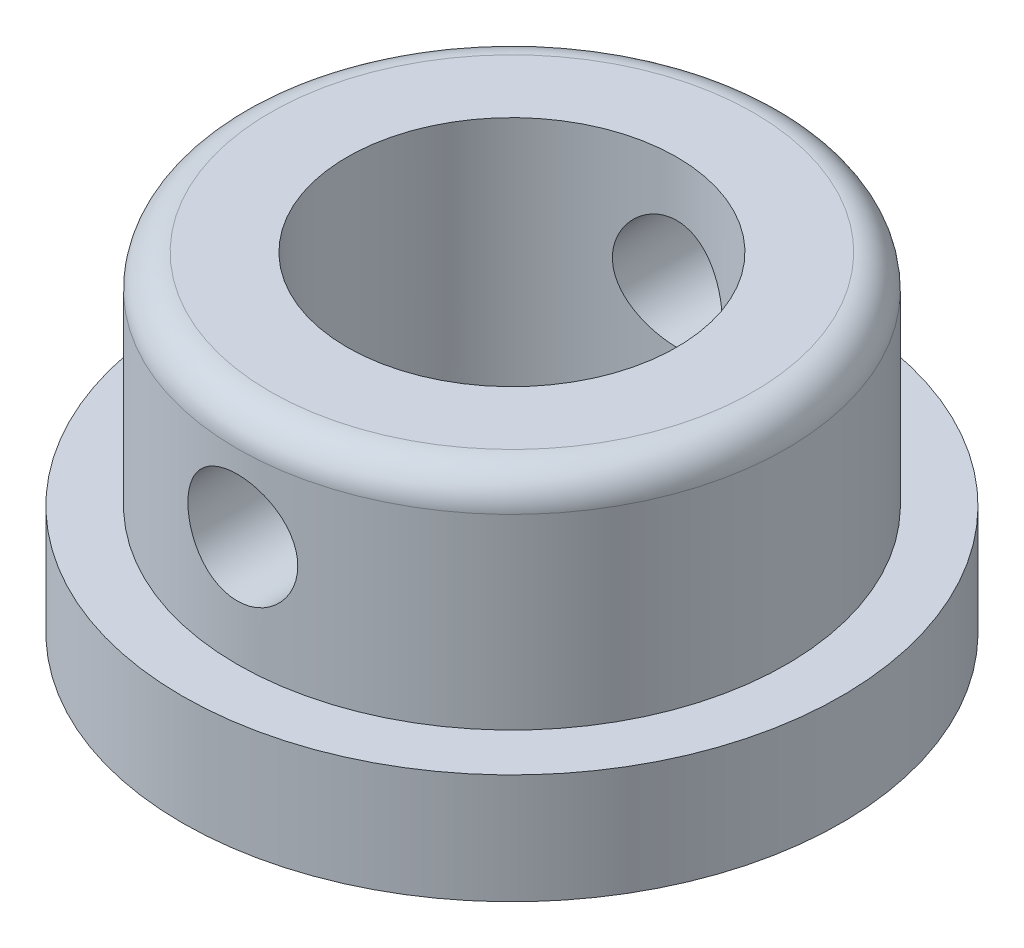
ISO-10303-21;
HEADER;
FILE_DESCRIPTION(('STEP AP214'),'2;1');
FILE_NAME('part.step','',(''),(''),'','','');
FILE_SCHEMA(('AUTOMOTIVE_DESIGN { 1 0 10303 214 1 1 1 1 }'));
ENDSEC;
DATA;
#1=APPLICATION_CONTEXT('core data for automotive mechanical design processes');
#2=APPLICATION_PROTOCOL_DEFINITION('international standard','automotive_design',2000,#1);
#3=PRODUCT_CONTEXT('',#1,'mechanical');
#4=PRODUCT('Part','Part','',(#3));
#5=PRODUCT_RELATED_PRODUCT_CATEGORY('part','',(#4));
#6=PRODUCT_DEFINITION_FORMATION('','',#4);
#7=PRODUCT_DEFINITION_CONTEXT('part definition',#1,'design');
#8=PRODUCT_DEFINITION('design','',#6,#7);
#9=PRODUCT_DEFINITION_SHAPE('','',#8);
#10=(LENGTH_UNIT() NAMED_UNIT(*) SI_UNIT(.MILLI.,.METRE.));
#11=(NAMED_UNIT(*) PLANE_ANGLE_UNIT() SI_UNIT($,.RADIAN.));
#12=(NAMED_UNIT(*) SI_UNIT($,.STERADIAN.) SOLID_ANGLE_UNIT());
#13=UNCERTAINTY_MEASURE_WITH_UNIT(LENGTH_MEASURE(1.E-05),#10,'distance_accuracy_value','');
#14=(GEOMETRIC_REPRESENTATION_CONTEXT(3) GLOBAL_UNCERTAINTY_ASSIGNED_CONTEXT((#13)) GLOBAL_UNIT_ASSIGNED_CONTEXT((#10,
#11,#12)) REPRESENTATION_CONTEXT('',''));
#15=CARTESIAN_POINT('',(0.,0.,0.));
#16=DIRECTION('',(0.,0.,1.));
#17=DIRECTION('',(1.,0.,0.));
#18=AXIS2_PLACEMENT_3D('',#15,#16,#17);
#19=CARTESIAN_POINT('',(0.,20.,-35.));
#20=DIRECTION('',(0.,0.,1.));
#21=DIRECTION('',(1.,0.,0.));
#22=AXIS2_PLACEMENT_3D('',#19,#20,#21);
#23=CYLINDRICAL_SURFACE('',#22,5.);
#24=CARTESIAN_POINT('',(5.,20.,-14.142135623731));
#25=CARTESIAN_POINT('',(5.00000128973857,20.2723408741804,-14.1421347265217));
#26=CARTESIAN_POINT('',(4.97767391842761,20.544673999118,-14.1500884645429));
#27=CARTESIAN_POINT('',(4.88925565844404,21.0812721049712,-14.1808787040627));
#28=CARTESIAN_POINT('',(4.82315756084199,21.3455357493623,-14.2037176571094));
#29=CARTESIAN_POINT('',(4.64977742842453,21.8581344649864,-14.2614101844396));
#30=CARTESIAN_POINT('',(4.54257610701623,22.1064996472136,-14.2962401985661));
#31=CARTESIAN_POINT('',(4.29030814220691,22.5818002427398,-14.3739561005162));
#32=CARTESIAN_POINT('',(4.14523314430092,22.8087309127682,-14.4168437651806));
#33=CARTESIAN_POINT('',(3.81525573221439,23.2435998116916,-14.5077244703737));
#34=CARTESIAN_POINT('',(3.6291217068896,23.4505771433586,-14.5558447422322));
#35=CARTESIAN_POINT('',(3.22493833607198,23.8310340061232,-14.6506932400501));
#36=CARTESIAN_POINT('',(3.00688387526188,24.0045081579118,-14.6974212414481));
#37=CARTESIAN_POINT('',(2.53802253982505,24.317394486648,-14.7856933460899));
#38=CARTESIAN_POINT('',(2.28650955612262,24.4557998530898,-14.8270703850803));
#39=CARTESIAN_POINT('',(1.76215611493737,24.6879579256375,-14.8984793385491));
#40=CARTESIAN_POINT('',(1.48932142843606,24.7817226658845,-14.9285143101501));
#41=CARTESIAN_POINT('',(0.940144087167472,24.918679273162,-14.9729537715953));
#42=CARTESIAN_POINT('',(0.664253774264842,24.963517231285,-14.987865738878));
#43=CARTESIAN_POINT('',(0.108489374120447,25.0065814668033,-15.0021804109124));
#44=CARTESIAN_POINT('',(-0.171383667719483,25.0048197582621,-15.0015871131448));
#45=CARTESIAN_POINT('',(-0.715517575969074,24.9557787271699,-14.9853019809366));
#46=CARTESIAN_POINT('',(-0.979960242958283,24.9102873576276,-14.9702032377559));
#47=CARTESIAN_POINT('',(-1.49721719411086,24.7780350950976,-14.9273483669866));
#48=CARTESIAN_POINT('',(-1.75003068889608,24.6912714051009,-14.8995913815591));
#49=CARTESIAN_POINT('',(-2.24076237420987,24.4778934134697,-14.8337835146612));
#50=CARTESIAN_POINT('',(-2.47844110484423,24.3507703072674,-14.7956021262008));
#51=CARTESIAN_POINT('',(-2.92962162763661,24.0607014727567,-14.712919651946));
#52=CARTESIAN_POINT('',(-3.14311667192671,23.8977457833618,-14.6684168100733));
#53=CARTESIAN_POINT('',(-3.55050433275654,23.5316280327015,-14.5753095924948));
#54=CARTESIAN_POINT('',(-3.74300078532636,23.3269342107926,-14.5266107584439));
#55=CARTESIAN_POINT('',(-4.09138629799087,22.8877563713669,-14.432366762445));
#56=CARTESIAN_POINT('',(-4.24726971640772,22.6532677713598,-14.3868220872808));
#57=CARTESIAN_POINT('',(-4.51993727517872,22.1567318719828,-14.3035262560556));
#58=CARTESIAN_POINT('',(-4.6361323181067,21.8943393434111,-14.2658954642374));
#59=CARTESIAN_POINT('',(-4.82221596634668,21.3521430289279,-14.2040825412192));
#60=CARTESIAN_POINT('',(-4.89212397873747,21.0723465939688,-14.1798947743546));
#61=CARTESIAN_POINT('',(-4.98080641048761,20.5168082229421,-14.1489818157793));
#62=CARTESIAN_POINT('',(-5.00174547753816,20.2414528762567,-14.1415180159378));
#63=CARTESIAN_POINT('',(-4.9980271945486,19.6911192544295,-14.1428336029592));
#64=CARTESIAN_POINT('',(-4.97337812613382,19.4161409198801,-14.1516100395907));
#65=CARTESIAN_POINT('',(-4.88112825776155,18.8842151714404,-14.183680904515));
#66=CARTESIAN_POINT('',(-4.81503196990342,18.6269728492458,-14.206466272042));
#67=CARTESIAN_POINT('',(-4.64356931280233,18.1272819688041,-14.2634276835511));
#68=CARTESIAN_POINT('',(-4.53819598181711,17.8848360420461,-14.297605746742));
#69=CARTESIAN_POINT('',(-4.28737170369468,17.413097895765,-14.3748438797893));
#70=CARTESIAN_POINT('',(-4.14075559179248,17.184466786791,-14.4181512832814));
#71=CARTESIAN_POINT('',(-3.81292815278779,16.7542697380814,-14.5082884365483));
#72=CARTESIAN_POINT('',(-3.63170662749391,16.5527118066939,-14.5551192221897));
#73=CARTESIAN_POINT('',(-3.22945852950163,16.1723600795468,-14.6497519318925));
#74=CARTESIAN_POINT('',(-3.00693635273326,15.9951280499057,-14.6974921788948));
#75=CARTESIAN_POINT('',(-2.53413645700128,15.6804192882598,-14.7863425806554));
#76=CARTESIAN_POINT('',(-2.28385972432276,15.5429411441879,-14.8274529708847));
#77=CARTESIAN_POINT('',(-1.76389931216148,15.3128994756914,-14.8982202905301));
#78=CARTESIAN_POINT('',(-1.49435561660598,15.2200436142597,-14.9279515002266));
#79=CARTESIAN_POINT('',(-0.942292329230079,15.0813612896995,-14.9729305418887));
#80=CARTESIAN_POINT('',(-0.659777459769445,15.0355178505975,-14.9881836017009));
#81=CARTESIAN_POINT('',(-0.104076679300203,14.9936896119718,-15.0020931618128));
#82=CARTESIAN_POINT('',(0.168923619600093,14.9954627303381,-15.001496004472));
#83=CARTESIAN_POINT('',(0.71055572500087,15.043286540732,-14.9856098259699));
#84=CARTESIAN_POINT('',(0.979187884095285,15.0893336407638,-14.9703219966788));
#85=CARTESIAN_POINT('',(1.5002105971603,15.2229111728798,-14.9270457477206));
#86=CARTESIAN_POINT('',(1.75279135456395,15.3097710767647,-14.8992629180574));
#87=CARTESIAN_POINT('',(2.23989175469898,15.5218876554858,-14.8338580352247));
#88=CARTESIAN_POINT('',(2.47440812071216,15.6471512759851,-14.7962342024008));
#89=CARTESIAN_POINT('',(2.92817008154393,15.93784756051,-14.713293441394));
#90=CARTESIAN_POINT('',(3.14653125778804,16.1045934269082,-14.6677436245963));
#91=CARTESIAN_POINT('',(3.55290513136214,16.471286955781,-14.574649439594));
#92=CARTESIAN_POINT('',(3.74090810812296,16.6712452113136,-14.5271044386549));
#93=CARTESIAN_POINT('',(4.08870904416559,17.1080467779347,-14.4331639912799));
#94=CARTESIAN_POINT('',(4.2471148299895,17.3460275548832,-14.3868863994315));
#95=CARTESIAN_POINT('',(4.52157171650558,17.8466721345139,-14.3030096661508));
#96=CARTESIAN_POINT('',(4.63763388409737,18.1093294651483,-14.2654082580625));
#97=CARTESIAN_POINT('',(4.81921914102083,18.6398091200782,-14.2050667103257));
#98=CARTESIAN_POINT('',(4.8867895457476,18.9068613176268,-14.1817316428591));
#99=CARTESIAN_POINT('',(4.97717160074634,19.4492802523335,-14.1502691769759));
#100=CARTESIAN_POINT('',(4.99999869598296,19.7246440870535,-14.1421365308731));
#101=CARTESIAN_POINT('',(5.,20.,-14.142135623731));
#102=B_SPLINE_CURVE_WITH_KNOTS('',3,(#24,#25,#26,#27,#28,#29,#30,#31,#32,#33,#34,#35,#36,#37,
#38,#39,#40,#41,#42,#43,#44,#45,#46,#47,#48,#49,#50,#51,#52,#53,#54,#55,#56,#57,#58,#59,#60,#61,
#62,#63,#64,#65,#66,#67,#68,#69,#70,#71,#72,#73,#74,#75,#76,#77,#78,#79,#80,#81,#82,#83,#84,#85,
#86,#87,#88,#89,#90,#91,#92,#93,#94,#95,#96,#97,#98,#99,#100,#101),.UNSPECIFIED.,.T.,.F.,(4,2,2,
2,2,2,2,2,2,2,2,2,2,2,2,2,2,2,2,2,2,2,2,2,2,2,2,2,2,2,2,2,2,2,2,2,2,2,4),(0.,0.816002923996784,
1.63214027507582,2.44668313750414,3.26140583092721,4.1050668713784,4.9488632585994,
5.81467530718286,6.68025381933945,7.51571593824671,8.35096266511636,9.15345024127845,
9.95599220946183,10.7690827430168,11.5823995937011,12.4340087181959,13.2857489806053,
14.1496319921528,15.0131525678308,15.837714568222,16.6621267918617,17.4582197884388,
18.2544539573473,19.0759428867857,19.8976742831064,20.7589404085546,21.6201759378766,
22.4756895595426,23.3308941502078,24.1459042338818,24.9608482004891,25.7628478020215,
26.5649925381621,27.3967759760317,28.2288252216316,29.0934451368072,29.9578389133433,
30.7831606081345,31.6081973595232),.UNSPECIFIED.);
#103=CARTESIAN_POINT('',(5.,20.,-14.142135623731));
#104=VERTEX_POINT('',#103);
#105=EDGE_CURVE('E50',#104,#104,#102,.T.);
#106=ORIENTED_EDGE('',*,*,#105,.T.);
#107=EDGE_LOOP('',(#106));
#108=FACE_BOUND('',#107,.T.);
#109=CARTESIAN_POINT('',(0.,25.,-25.));
#110=CARTESIAN_POINT('',(-0.138987493787324,25.0000027694463,-25.0000014065203));
#111=CARTESIAN_POINT('',(-0.277940302046088,24.9942032492811,-24.9988389427216));
#112=CARTESIAN_POINT('',(-0.554886864496204,24.9710563512974,-24.994224565157));
#113=CARTESIAN_POINT('',(-0.692880432791919,24.9537067948975,-24.9907722194715));
#114=CARTESIAN_POINT('',(-0.966937148503881,24.9075814377122,-24.981670242636));
#115=CARTESIAN_POINT('',(-1.10299928122357,24.8787998455141,-24.9760194978176));
#116=CARTESIAN_POINT('',(-1.37221108352448,24.810025349109,-24.9626762565998));
#117=CARTESIAN_POINT('',(-1.50535966309261,24.7700283237777,-24.9549830097359));
#118=CARTESIAN_POINT('',(-1.76758319373794,24.6791962522582,-24.9377804442932));
#119=CARTESIAN_POINT('',(-1.896663374225,24.6283758297848,-24.9282735779222));
#120=CARTESIAN_POINT('',(-2.15009997814349,24.5162240178123,-24.9076944208426));
#121=CARTESIAN_POINT('',(-2.2744546389337,24.4548887523412,-24.8966215531404));
#122=CARTESIAN_POINT('',(-2.51749782000809,24.3221945692906,-24.8732206370355));
#123=CARTESIAN_POINT('',(-2.63618884664852,24.2508401417061,-24.8608931515555));
#124=CARTESIAN_POINT('',(-2.86722020463686,24.0985603647523,-24.8353088041128));
#125=CARTESIAN_POINT('',(-2.97955814193969,24.0176314424647,-24.8220515959613));
#126=CARTESIAN_POINT('',(-3.1983785388143,23.8457711931702,-24.7948114657324));
#127=CARTESIAN_POINT('',(-3.30477652475173,23.7547333566458,-24.780821838943));
#128=CARTESIAN_POINT('',(-3.50958996762926,23.5640376679645,-24.7526457290753));
#129=CARTESIAN_POINT('',(-3.60800245195942,23.4643766340819,-24.738459174971));
#130=CARTESIAN_POINT('',(-3.79610927604841,23.2571655640739,-24.7102933832022));
#131=CARTESIAN_POINT('',(-3.8858061217282,23.1496178112366,-24.6963140869323));
#132=CARTESIAN_POINT('',(-4.05592901668139,22.9272928345424,-24.6689453876667));
#133=CARTESIAN_POINT('',(-4.13635163435981,22.8125129588355,-24.6555562041458));
#134=CARTESIAN_POINT('',(-4.28798741229219,22.5754841568505,-24.6296394657581));
#135=CARTESIAN_POINT('',(-4.35911381454495,22.4531786550123,-24.6171204770982));
#136=CARTESIAN_POINT('',(-4.49081269831453,22.2028712528765,-24.5934353082732));
#137=CARTESIAN_POINT('',(-4.55138122040544,22.0748672380124,-24.5822696361062));
#138=CARTESIAN_POINT('',(-4.71644727257975,21.6837416438572,-24.5513304070068));
#139=CARTESIAN_POINT('',(-4.8044888260482,21.4132193246056,-24.5340820165952));
#140=CARTESIAN_POINT('',(-4.93264780265691,20.8645385652061,-24.508635793463));
#141=CARTESIAN_POINT('',(-4.97337819482264,20.5865266702931,-24.5003223072134));
#142=CARTESIAN_POINT('',(-5.00775493418216,20.027461501124,-24.4933199482487));
#143=CARTESIAN_POINT('',(-5.00140609582258,19.7464085407904,-24.4946300913956));
#144=CARTESIAN_POINT('',(-4.94227436036826,19.1937632800715,-24.5066272442008));
#145=CARTESIAN_POINT('',(-4.89019310186595,18.9220922268258,-24.5171725589932));
#146=CARTESIAN_POINT('',(-4.7421890224497,18.3914203617583,-24.546227391949));
#147=CARTESIAN_POINT('',(-4.64626410780486,18.1324201556801,-24.5647372904543));
#148=CARTESIAN_POINT('',(-4.41262402680007,17.6324234898532,-24.6077809023025));
#149=CARTESIAN_POINT('',(-4.27463078523214,17.3915605480925,-24.632354484594));
#150=CARTESIAN_POINT('',(-3.96096784378848,16.9361458042038,-24.684730944745));
#151=CARTESIAN_POINT('',(-3.78529381392921,16.721597030353,-24.7125341935642));
#152=CARTESIAN_POINT('',(-3.39749968079915,16.3208529728437,-24.7688510603976));
#153=CARTESIAN_POINT('',(-3.18478080820446,16.1352371567135,-24.797368460096));
#154=CARTESIAN_POINT('',(-2.73092511816778,15.8022307724848,-24.8514424361697));
#155=CARTESIAN_POINT('',(-2.48978793632426,15.654840694624,-24.8769989745701));
#156=CARTESIAN_POINT('',(-1.98529693496818,15.4023624527765,-24.9223345079227));
#157=CARTESIAN_POINT('',(-1.72190909807365,15.2973405314029,-24.9421044423773));
#158=CARTESIAN_POINT('',(-1.18074488209619,15.1331976301815,-24.9735704494292));
#159=CARTESIAN_POINT('',(-0.9029702503472,15.0740710900358,-24.98526750005));
#160=CARTESIAN_POINT('',(-0.34589702815055,15.0042177306314,-24.9991335933204));
#161=CARTESIAN_POINT('',(-0.0667016415443239,14.9926979010851,-25.0014587325673));
#162=CARTESIAN_POINT('',(0.489624670880016,15.0162492959244,-24.9967525965614));
#163=CARTESIAN_POINT('',(0.766755711869967,15.0513179012196,-24.9897218472742));
#164=CARTESIAN_POINT('',(1.30852830007857,15.1663918633032,-24.9671916002008));
#165=CARTESIAN_POINT('',(1.57325974299468,15.2459903260944,-24.9517688194687));
#166=CARTESIAN_POINT('',(2.08561813620307,15.4474199296754,-24.9141776037933));
#167=CARTESIAN_POINT('',(2.33324380335236,15.5692542345549,-24.892008663478));
#168=CARTESIAN_POINT('',(2.80770587332562,15.853412391337,-24.8429955738642));
#169=CARTESIAN_POINT('',(3.03425065213174,16.0162136728006,-24.8160975113418));
#170=CARTESIAN_POINT('',(3.45709007722326,16.3770461884555,-24.760736752006));
#171=CARTESIAN_POINT('',(3.65338147605435,16.5750811997927,-24.7322738876682));
#172=CARTESIAN_POINT('',(4.01320302351496,17.0043658784477,-24.6764651380018));
#173=CARTESIAN_POINT('',(4.17618877400404,17.2360754097949,-24.6491428619003));
#174=CARTESIAN_POINT('',(4.46092683850573,17.7240601179627,-24.5992097395686));
#175=CARTESIAN_POINT('',(4.58268080227279,17.9803343113826,-24.5765987048474));
#176=CARTESIAN_POINT('',(4.78076018011429,18.5088289322538,-24.5388364729789));
#177=CARTESIAN_POINT('',(4.85732111853824,18.7809584178571,-24.5236466726876));
#178=CARTESIAN_POINT('',(4.96353963899985,19.3347130495845,-24.5023739077135));
#179=CARTESIAN_POINT('',(4.9932033375265,19.6163369525221,-24.4962897554484));
#180=CARTESIAN_POINT('',(5.00179339144585,20.0366703889551,-24.4945288792509));
#181=CARTESIAN_POINT('',(4.99885021968412,20.1752265681492,-24.4951330184965));
#182=CARTESIAN_POINT('',(4.98148651470878,20.4515737957145,-24.4986714739674));
#183=CARTESIAN_POINT('',(4.9670703371849,20.5893651144752,-24.5016049058833));
#184=CARTESIAN_POINT('',(4.92686276339316,20.8632490159191,-24.5097212135577));
#185=CARTESIAN_POINT('',(4.90106738632089,20.9993409869687,-24.5149048765081));
#186=CARTESIAN_POINT('',(4.83831799577184,21.2687799057397,-24.5273664043086));
#187=CARTESIAN_POINT('',(4.80136796328246,21.402127814684,-24.5346435219816));
#188=CARTESIAN_POINT('',(4.71667811844351,21.6649227005665,-24.5510651803018));
#189=CARTESIAN_POINT('',(4.66896100938054,21.7943772453011,-24.5602057877658));
#190=CARTESIAN_POINT('',(4.56306801677477,22.0487516964052,-24.5800998692381));
#191=CARTESIAN_POINT('',(4.5048958336854,22.1736731884551,-24.5908527723703));
#192=CARTESIAN_POINT('',(4.37847423732261,22.4182475627271,-24.6136768592635));
#193=CARTESIAN_POINT('',(4.31022064232977,22.537898231772,-24.6257485895239));
#194=CARTESIAN_POINT('',(4.1641570153785,22.7710492454946,-24.6508678052533));
#195=CARTESIAN_POINT('',(4.08635026305033,22.8845516817026,-24.6639149552593));
#196=CARTESIAN_POINT('',(3.92025868558202,23.1066267352987,-24.6908640955351));
#197=CARTESIAN_POINT('',(3.83181538764857,23.2150795397072,-24.7047769949563));
#198=CARTESIAN_POINT('',(3.64620484015059,23.424138296357,-24.7328525343466));
#199=CARTESIAN_POINT('',(3.54904066604526,23.5247469916541,-24.7470150848702));
#200=CARTESIAN_POINT('',(3.34655721556743,23.717540620803,-24.7752095204235));
#201=CARTESIAN_POINT('',(3.24123314471885,23.8097205317761,-24.7892413231228));
#202=CARTESIAN_POINT('',(3.02322778921367,23.9849269400267,-24.8167717117019));
#203=CARTESIAN_POINT('',(2.91054922625043,24.067956793247,-24.8302704919035));
#204=CARTESIAN_POINT('',(2.67729343786965,24.2251738971151,-24.8565085935593));
#205=CARTESIAN_POINT('',(2.55664367436167,24.2992552310598,-24.869238066002));
#206=CARTESIAN_POINT('',(2.30944481023433,24.4369443352167,-24.8934104051449));
#207=CARTESIAN_POINT('',(2.18289789785573,24.5005559513136,-24.9048537437938));
#208=CARTESIAN_POINT('',(1.9248233263731,24.6168245035003,-24.9261268452451));
#209=CARTESIAN_POINT('',(1.79329873940675,24.6694880703005,-24.9359575839567));
#210=CARTESIAN_POINT('',(1.5261844247676,24.763487680713,-24.9537310452209));
#211=CARTESIAN_POINT('',(1.39059548585458,24.8048259066209,-24.9616741314688));
#212=CARTESIAN_POINT('',(1.04920215690347,24.8932231271974,-24.9788087281562));
#213=CARTESIAN_POINT('',(0.841457494405877,24.9332098107155,-24.9867141903289));
#214=CARTESIAN_POINT('',(0.422448453280689,24.9865957194188,-24.9973086745575));
#215=CARTESIAN_POINT('',(0.211184187046264,24.9999957919719,-24.9999978628663));
#216=CARTESIAN_POINT('',(0.,25.,-25.));
#217=B_SPLINE_CURVE_WITH_KNOTS('',3,(#109,#110,#111,#112,#113,#114,#115,#116,#117,#118,#119,
#120,#121,#122,#123,#124,#125,#126,#127,#128,#129,#130,#131,#132,#133,#134,#135,#136,#137,#138,
#139,#140,#141,#142,#143,#144,#145,#146,#147,#148,#149,#150,#151,#152,#153,#154,#155,#156,#157,
#158,#159,#160,#161,#162,#163,#164,#165,#166,#167,#168,#169,#170,#171,#172,#173,#174,#175,#176,
#177,#178,#179,#180,#181,#182,#183,#184,#185,#186,#187,#188,#189,#190,#191,#192,#193,#194,#195,
#196,#197,#198,#199,#200,#201,#202,#203,#204,#205,#206,#207,#208,#209,#210,#211,#212,#213,#214,
#215,#216),.UNSPECIFIED.,.T.,.F.,(4,2,2,2,2,2,2,2,2,2,2,2,2,2,2,2,2,2,2,2,2,2,2,2,2,2,2,2,2,2,2,
2,2,2,2,2,2,2,2,2,2,2,2,2,2,2,2,2,2,2,2,2,2,4),(0.,0.416777047445418,0.833632730149863,
1.25069985977206,1.66792044248879,2.0845808461562,2.50139517036218,2.91802329572165,
3.33480738770838,3.7564966440872,4.17834216132244,4.60006602836891,5.02194544187045,
5.44751701120413,5.87324783701269,6.72369555497644,7.56299734191929,8.40221330082507,
9.22877443707773,10.0553750494503,10.8875625969434,11.7198458242473,12.5671007113313,
13.4143664637548,14.262951829465,15.1114343716656,15.9457248705771,16.7799684696572,
17.6067107843,18.4335150475649,19.2704413884317,20.1074575040603,20.9572195157251,
21.8069475229371,22.6522071384191,23.4973565033242,23.9127168808878,24.3279196434016,
24.7432677723233,25.1584678424529,25.5728004765726,25.9869867501795,26.4013453111814,
26.8155620171985,27.2369706991647,27.6582313488923,28.0797414220244,28.5010963808509,
28.9270309561325,29.3528087202144,29.7783278548953,30.203764937947,30.8370559265658,
31.4703267306209),.UNSPECIFIED.);
#218=CARTESIAN_POINT('',(0.,25.,-25.));
#219=VERTEX_POINT('',#218);
#220=EDGE_CURVE('E75',#219,#219,#217,.T.);
#221=ORIENTED_EDGE('',*,*,#220,.F.);
#222=EDGE_LOOP('',(#221));
#223=FACE_BOUND('',#222,.T.);
#224=ADVANCED_FACE('F43',(#108,#223),#23,.F.);
#225=CARTESIAN_POINT('',(0.,10.,0.));
#226=DIRECTION('',(0.,-1.,0.));
#227=DIRECTION('',(0.,0.,-1.));
#228=AXIS2_PLACEMENT_3D('',#225,#226,#227);
#229=CYLINDRICAL_SURFACE('',#228,30.);
#230=CARTESIAN_POINT('',(0.,10.,0.));
#231=DIRECTION('',(0.,1.,0.));
#232=DIRECTION('',(0.,0.,1.));
#233=AXIS2_PLACEMENT_3D('',#230,#231,#232);
#234=CIRCLE('',#233,30.);
#235=CARTESIAN_POINT('',(0.,10.,30.));
#236=VERTEX_POINT('',#235);
#237=EDGE_CURVE('E128',#236,#236,#234,.T.);
#238=ORIENTED_EDGE('',*,*,#237,.F.);
#239=EDGE_LOOP('',(#238));
#240=FACE_BOUND('',#239,.T.);
#241=CARTESIAN_POINT('',(0.,0.,0.));
#242=DIRECTION('',(0.,1.,0.));
#243=DIRECTION('',(0.,0.,1.));
#244=AXIS2_PLACEMENT_3D('',#241,#242,#243);
#245=CIRCLE('',#244,30.);
#246=CARTESIAN_POINT('',(0.,0.,30.));
#247=VERTEX_POINT('',#246);
#248=EDGE_CURVE('E126',#247,#247,#245,.T.);
#249=ORIENTED_EDGE('',*,*,#248,.T.);
#250=EDGE_LOOP('',(#249));
#251=FACE_BOUND('',#250,.T.);
#252=ADVANCED_FACE('F113',(#240,#251),#229,.T.);
#253=CARTESIAN_POINT('',(0.,10.,0.));
#254=DIRECTION('',(0.,1.,0.));
#255=DIRECTION('',(0.,0.,1.));
#256=AXIS2_PLACEMENT_3D('',#253,#254,#255);
#257=PLANE('',#256);
#258=CARTESIAN_POINT('',(0.,10.,0.));
#259=DIRECTION('',(0.,1.,0.));
#260=DIRECTION('',(0.,0.,1.));
#261=AXIS2_PLACEMENT_3D('',#258,#259,#260);
#262=CIRCLE('',#261,25.);
#263=CARTESIAN_POINT('',(0.,10.,25.));
#264=VERTEX_POINT('',#263);
#265=EDGE_CURVE('E61',#264,#264,#262,.T.);
#266=ORIENTED_EDGE('',*,*,#265,.F.);
#267=EDGE_LOOP('',(#266));
#268=FACE_BOUND('',#267,.T.);
#269=ORIENTED_EDGE('',*,*,#237,.T.);
#270=EDGE_LOOP('',(#269));
#271=FACE_BOUND('',#270,.T.);
#272=ADVANCED_FACE('F120',(#268,#271),#257,.T.);
#273=CARTESIAN_POINT('',(0.,0.,0.));
#274=DIRECTION('',(0.,1.,0.));
#275=DIRECTION('',(0.,0.,1.));
#276=AXIS2_PLACEMENT_3D('',#273,#274,#275);
#277=PLANE('',#276);
#278=CARTESIAN_POINT('',(0.,0.,0.));
#279=DIRECTION('',(0.,-1.,0.));
#280=DIRECTION('',(0.,0.,-1.));
#281=AXIS2_PLACEMENT_3D('',#278,#279,#280);
#282=CIRCLE('',#281,25.);
#283=CARTESIAN_POINT('',(0.,0.,-25.));
#284=VERTEX_POINT('',#283);
#285=EDGE_CURVE('E138',#284,#284,#282,.T.);
#286=ORIENTED_EDGE('',*,*,#285,.F.);
#287=EDGE_LOOP('',(#286));
#288=FACE_BOUND('',#287,.T.);
#289=ORIENTED_EDGE('',*,*,#248,.F.);
#290=EDGE_LOOP('',(#289));
#291=FACE_BOUND('',#290,.T.);
#292=ADVANCED_FACE('F172',(#288,#291),#277,.F.);
#293=CARTESIAN_POINT('',(0.,30.,0.));
#294=DIRECTION('',(0.,-1.,0.));
#295=DIRECTION('',(0.,0.,-1.));
#296=AXIS2_PLACEMENT_3D('',#293,#294,#295);
#297=CYLINDRICAL_SURFACE('',#296,25.);
#298=ORIENTED_EDGE('',*,*,#220,.T.);
#299=EDGE_LOOP('',(#298));
#300=FACE_BOUND('',#299,.T.);
#301=CARTESIAN_POINT('',(5.,20.,24.4948974278318));
#302=CARTESIAN_POINT('',(5.00000277932283,19.8610437715678,24.4948959140652));
#303=CARTESIAN_POINT('',(4.99420583952395,19.722122240573,24.4960820445244));
#304=CARTESIAN_POINT('',(4.97106951247274,19.4452390892176,24.5007881327193));
#305=CARTESIAN_POINT('',(4.95372794446977,19.307277655193,24.5043085313918));
#306=CARTESIAN_POINT('',(4.90762442723258,19.0332858709187,24.5135833999899));
#307=CARTESIAN_POINT('',(4.8788566379347,18.8972565450725,24.5193390123237));
#308=CARTESIAN_POINT('',(4.8101161975473,18.6281110791934,24.5329168521693));
#309=CARTESIAN_POINT('',(4.77013942141009,18.4949960311311,24.5407398404405));
#310=CARTESIAN_POINT('',(4.679356239882,18.2328438594748,24.5582115919251));
#311=CARTESIAN_POINT('',(4.62856486213673,18.1038013596023,24.5678578195523));
#312=CARTESIAN_POINT('',(4.51647818958425,17.8504369587209,24.5887102826167));
#313=CARTESIAN_POINT('',(4.45517901998884,17.7261168198334,24.5999170932378));
#314=CARTESIAN_POINT('',(4.32256259117468,17.4831366609698,24.6235656382957));
#315=CARTESIAN_POINT('',(4.25124978528394,17.3644741561491,24.6360068230559));
#316=CARTESIAN_POINT('',(4.09905714012307,17.1334921966877,24.6617859698465));
#317=CARTESIAN_POINT('',(4.01817372862809,17.0211751337375,24.6751242659164));
#318=CARTESIAN_POINT('',(3.84635941756608,16.8023273728514,24.7024933301151));
#319=CARTESIAN_POINT('',(3.7553169869603,16.6958850347564,24.7165306060046));
#320=CARTESIAN_POINT('',(3.56460271884441,16.4909823888348,24.7447550172108));
#321=CARTESIAN_POINT('',(3.46492769556318,16.3925250539721,24.7589422061409));
#322=CARTESIAN_POINT('',(3.25767968751707,16.2043303455565,24.7870621737417));
#323=CARTESIAN_POINT('',(3.15010904621878,16.114590402856,24.80099502638));
#324=CARTESIAN_POINT('',(2.92772937682516,15.9443844675538,24.8282290266689));
#325=CARTESIAN_POINT('',(2.81291769594009,15.8639219046559,24.8415299396397));
#326=CARTESIAN_POINT('',(2.57586269555548,15.7122400706679,24.867232331661));
#327=CARTESIAN_POINT('',(2.45356521066841,15.6411038142726,24.8796253494226));
#328=CARTESIAN_POINT('',(2.20327286170084,15.5093843802369,24.9030409030999));
#329=CARTESIAN_POINT('',(2.0752758829805,15.4488051611513,24.9140629244939));
#330=CARTESIAN_POINT('',(1.68417147036292,15.2837064735327,24.9445697433125));
#331=CARTESIAN_POINT('',(1.4136645417639,15.1956431521847,24.9615274484324));
#332=CARTESIAN_POINT('',(0.865044260538017,15.0674427049637,24.9865205281948));
#333=CARTESIAN_POINT('',(0.587078089251455,15.0266894005891,24.9946705178815));
#334=CARTESIAN_POINT('',(0.0281034479881197,14.9922509518139,25.001544855821));
#335=CARTESIAN_POINT('',(-0.252904726222845,14.9985612718641,25.0002701123409));
#336=CARTESIAN_POINT('',(-0.805712786453449,15.0576294026319,24.9885220591615));
#337=CARTESIAN_POINT('',(-1.07758681729646,15.1097244842391,24.9781800029126));
#338=CARTESIAN_POINT('',(-1.60865738706756,15.2578255639107,24.9496087733464));
#339=CARTESIAN_POINT('',(-1.86785341829838,15.3538333188906,24.93137928446));
#340=CARTESIAN_POINT('',(-2.36809751770485,15.5876500921249,24.8888648238832));
#341=CARTESIAN_POINT('',(-2.60902092474939,15.7257187264038,24.8645424148967));
#342=CARTESIAN_POINT('',(-3.06452517521266,16.039545415307,24.812523467553));
#343=CARTESIAN_POINT('',(-3.27910298301493,16.2153078067188,24.7848265411053));
#344=CARTESIAN_POINT('',(-3.67975717013202,16.603168102539,24.7285482199077));
#345=CARTESIAN_POINT('',(-3.86527158685728,16.8158459315038,24.6999598233212));
#346=CARTESIAN_POINT('',(-4.19809246189484,17.269582214398,24.6455785794926));
#347=CARTESIAN_POINT('',(-4.3453981975471,17.5106412049894,24.6197857851305));
#348=CARTESIAN_POINT('',(-4.5978140751034,18.0151041585344,24.5739023737433));
#349=CARTESIAN_POINT('',(-4.7028332392629,18.2785548380507,24.5538240781191));
#350=CARTESIAN_POINT('',(-4.86695170776361,18.8198566187675,24.521823816122));
#351=CARTESIAN_POINT('',(-4.9260569968798,19.0977058381111,24.5099007867518));
#352=CARTESIAN_POINT('',(-4.99583003057767,19.654824289987,24.4957739630664));
#353=CARTESIAN_POINT('',(-5.00730929570102,19.9339878716477,24.493407351626));
#354=CARTESIAN_POINT('',(-4.98368814034094,20.4902411159245,24.4982242831088));
#355=CARTESIAN_POINT('',(-4.94859036116145,20.7673308952462,24.5054072844901));
#356=CARTESIAN_POINT('',(-4.83351104478034,21.308843201799,24.5283616252697));
#357=CARTESIAN_POINT('',(-4.75396312055877,21.5733617164651,24.5440499515026));
#358=CARTESIAN_POINT('',(-4.55270516017896,22.0853163938573,24.5821744668054));
#359=CARTESIAN_POINT('',(-4.43099165081897,22.3327511473708,24.6046112117261));
#360=CARTESIAN_POINT('',(-4.1470207729206,22.8070655546213,24.6540703007231));
#361=CARTESIAN_POINT('',(-3.98425562210339,23.0336352497929,24.6811486029996));
#362=CARTESIAN_POINT('',(-3.62347762885004,23.4565415417139,24.7366861815763));
#363=CARTESIAN_POINT('',(-3.4254611586761,23.6528750229515,24.7651455997886));
#364=CARTESIAN_POINT('',(-2.99616224784609,24.0128128652711,24.8207673304219));
#365=CARTESIAN_POINT('',(-2.76441580370579,24.1758685338953,24.8479030243562));
#366=CARTESIAN_POINT('',(-2.27633617425512,24.4607291468636,24.8973562425148));
#367=CARTESIAN_POINT('',(-2.02000402205358,24.5825358235458,24.9196739690654));
#368=CARTESIAN_POINT('',(-1.49152568807435,24.7806453263062,24.9568652187611));
#369=CARTESIAN_POINT('',(-1.21947909079514,24.8572061926372,24.9717808767));
#370=CARTESIAN_POINT('',(-0.66590155550293,24.9634526372471,24.9926598775445));
#371=CARTESIAN_POINT('',(-0.384371763979328,24.9931438612975,24.9986242986841));
#372=CARTESIAN_POINT('',(0.0359308696076347,25.0018003890947,25.0003623098663));
#373=CARTESIAN_POINT('',(0.174547706902777,24.9988756420099,24.9997743264358));
#374=CARTESIAN_POINT('',(0.45101825034353,24.9815385408312,24.9963121932555));
#375=CARTESIAN_POINT('',(0.588872225946723,24.9671305434389,24.9934389105404));
#376=CARTESIAN_POINT('',(0.862882900616901,24.9269286368396,24.9854807163608));
#377=CARTESIAN_POINT('',(0.999038995028388,24.9011307841561,24.9803950389143));
#378=CARTESIAN_POINT('',(1.2686070645044,24.8383651655105,24.9681563049873));
#379=CARTESIAN_POINT('',(1.40202000237943,24.8014013926633,24.9610039876105));
#380=CARTESIAN_POINT('',(1.66496388536662,24.716666157964,24.9448434641995));
#381=CARTESIAN_POINT('',(1.79450185423182,24.6689157852204,24.9358388825964));
#382=CARTESIAN_POINT('',(2.04903823379664,24.5629420773169,24.9162142305196));
#383=CARTESIAN_POINT('',(2.17403823455953,24.5047224538994,24.9055947327996));
#384=CARTESIAN_POINT('',(2.4187611555957,24.378193382996,24.8830203693368));
#385=CARTESIAN_POINT('',(2.53848187993982,24.3098797873512,24.8710649550885));
#386=CARTESIAN_POINT('',(2.77176194719752,24.1636856073457,24.8461484673941));
#387=CARTESIAN_POINT('',(2.88532338962303,24.0858083128838,24.8331877403362));
#388=CARTESIAN_POINT('',(3.107409439357,23.9196372325023,24.8063847462598));
#389=CARTESIAN_POINT('',(3.21581998719232,23.831192745672,24.7925314606031));
#390=CARTESIAN_POINT('',(3.42479299282091,23.6455885973766,24.7645291791264));
#391=CARTESIAN_POINT('',(3.52535819417319,23.5484320083593,24.7503802888953));
#392=CARTESIAN_POINT('',(3.71806545178663,23.345972526609,24.7221657734697));
#393=CARTESIAN_POINT('',(3.81020243422066,23.2406647963557,24.7081002031371));
#394=CARTESIAN_POINT('',(3.98532502872243,23.0227010381552,24.6804587105912));
#395=CARTESIAN_POINT('',(4.06831398902585,22.9100477229278,24.6668826104611));
#396=CARTESIAN_POINT('',(4.22547700693866,22.6768148430827,24.6404498236186));
#397=CARTESIAN_POINT('',(4.29954219421514,22.5561607708029,24.6276028717508));
#398=CARTESIAN_POINT('',(4.43719880973621,22.3089555311573,24.6031736469171));
#399=CARTESIAN_POINT('',(4.50079408397347,22.1824065512268,24.5915909100867));
#400=CARTESIAN_POINT('',(4.61703044134767,21.9243288844637,24.5700331062172));
#401=CARTESIAN_POINT('',(4.6696782069991,21.792803293728,24.5600570592754));
#402=CARTESIAN_POINT('',(4.76364722951765,21.5256860019017,24.5420037041339));
#403=CARTESIAN_POINT('',(4.80497067776392,21.3900950931365,24.5339260286217));
#404=CARTESIAN_POINT('',(4.89330917087388,21.0487823116088,24.516494143671));
#405=CARTESIAN_POINT('',(4.9332633683589,20.841122048542,24.5084401426211));
#406=CARTESIAN_POINT('',(4.98660621384694,20.4222810828269,24.4976430260943));
#407=CARTESIAN_POINT('',(4.99999577768878,20.2111005017978,24.4948997275263));
#408=CARTESIAN_POINT('',(5.,20.,24.4948974278318));
#409=B_SPLINE_CURVE_WITH_KNOTS('',3,(#301,#302,#303,#304,#305,#306,#307,#308,#309,#310,#311,
#312,#313,#314,#315,#316,#317,#318,#319,#320,#321,#322,#323,#324,#325,#326,#327,#328,#329,#330,
#331,#332,#333,#334,#335,#336,#337,#338,#339,#340,#341,#342,#343,#344,#345,#346,#347,#348,#349,
#350,#351,#352,#353,#354,#355,#356,#357,#358,#359,#360,#361,#362,#363,#364,#365,#366,#367,#368,
#369,#370,#371,#372,#373,#374,#375,#376,#377,#378,#379,#380,#381,#382,#383,#384,#385,#386,#387,
#388,#389,#390,#391,#392,#393,#394,#395,#396,#397,#398,#399,#400,#401,#402,#403,#404,#405,#406,
#407,#408),.UNSPECIFIED.,.T.,.F.,(4,2,2,2,2,2,2,2,2,2,2,2,2,2,2,2,2,2,2,2,2,2,2,2,2,2,2,2,2,2,2,
2,2,2,2,2,2,2,2,2,2,2,2,2,2,2,2,2,2,2,2,2,2,4),(0.,0.416683123532559,0.833444979779735,
1.25042012213458,1.66754891843382,2.08410182437339,2.50080866752238,2.91733077366026,
3.33400883985332,3.75582155231458,4.17779059926178,4.59963490581338,5.02163466502477,
5.44716701587087,5.87285858614629,6.72323197660177,7.5624010084278,8.40148917008619,
9.22862804595065,10.0558000179613,10.8881847753889,11.7206653527771,12.5676559023979,
13.4146624704098,14.2634817229126,15.112190315075,15.9463764545252,16.780515290738,
17.6066556534829,18.4328640820369,19.269841553043,20.1069052078274,20.9568186509895,
21.8066963958222,22.6516792432494,23.4965602988983,23.9121012971265,24.3274847156826,
24.7430120641575,25.158390988859,25.5729647204247,25.9873917587991,26.4019895837877,
26.8164451851411,27.2377409358741,27.6588886906077,28.0802883323104,28.5015332232677,
28.9274855291216,29.3532810158644,29.7788158230356,30.2042682263315,30.8373096537297,
31.4703292560956),.UNSPECIFIED.);
#410=CARTESIAN_POINT('',(5.,20.,24.4948974278318));
#411=VERTEX_POINT('',#410);
#412=EDGE_CURVE('E65',#411,#411,#409,.T.);
#413=ORIENTED_EDGE('',*,*,#412,.T.);
#414=EDGE_LOOP('',(#413));
#415=FACE_BOUND('',#414,.T.);
#416=CARTESIAN_POINT('',(0.,27.,0.));
#417=DIRECTION('',(0.,1.,0.));
#418=DIRECTION('',(0.,0.,1.));
#419=AXIS2_PLACEMENT_3D('',#416,#417,#418);
#420=CIRCLE('',#419,25.);
#421=CARTESIAN_POINT('',(0.,27.,25.));
#422=VERTEX_POINT('',#421);
#423=EDGE_CURVE('E10',#422,#422,#420,.F.);
#424=ORIENTED_EDGE('',*,*,#423,.T.);
#425=EDGE_LOOP('',(#424));
#426=FACE_BOUND('',#425,.T.);
#427=ORIENTED_EDGE('',*,*,#265,.T.);
#428=EDGE_LOOP('',(#427));
#429=FACE_BOUND('',#428,.T.);
#430=ADVANCED_FACE('F77',(#300,#415,#426,#429),#297,.T.);
#431=CARTESIAN_POINT('',(0.,30.,0.));
#432=DIRECTION('',(0.,1.,0.));
#433=DIRECTION('',(0.,0.,1.));
#434=AXIS2_PLACEMENT_3D('',#431,#432,#433);
#435=PLANE('',#434);
#436=CARTESIAN_POINT('',(0.,30.,0.));
#437=DIRECTION('',(0.,1.,0.));
#438=DIRECTION('',(0.,0.,1.));
#439=AXIS2_PLACEMENT_3D('',#436,#437,#438);
#440=CIRCLE('',#439,15.);
#441=CARTESIAN_POINT('',(0.,30.,15.));
#442=VERTEX_POINT('',#441);
#443=EDGE_CURVE('E143',#442,#442,#440,.T.);
#444=ORIENTED_EDGE('',*,*,#443,.F.);
#445=EDGE_LOOP('',(#444));
#446=FACE_BOUND('',#445,.T.);
#447=CARTESIAN_POINT('',(0.,30.,0.));
#448=DIRECTION('',(0.,1.,0.));
#449=DIRECTION('',(0.,0.,1.));
#450=AXIS2_PLACEMENT_3D('',#447,#448,#449);
#451=CIRCLE('',#450,22.);
#452=CARTESIAN_POINT('',(0.,30.,22.));
#453=VERTEX_POINT('',#452);
#454=EDGE_CURVE('E57',#453,#453,#451,.T.);
#455=ORIENTED_EDGE('',*,*,#454,.T.);
#456=EDGE_LOOP('',(#455));
#457=FACE_BOUND('',#456,.T.);
#458=ADVANCED_FACE('F86',(#446,#457),#435,.T.);
#459=CARTESIAN_POINT('',(0.,27.,0.));
#460=DIRECTION('',(0.,1.,0.));
#461=DIRECTION('',(0.,0.,1.));
#462=AXIS2_PLACEMENT_3D('',#459,#460,#461);
#463=TOROIDAL_SURFACE('',#462,22.,3.);
#464=ORIENTED_EDGE('',*,*,#423,.F.);
#465=EDGE_LOOP('',(#464));
#466=FACE_BOUND('',#465,.T.);
#467=ORIENTED_EDGE('',*,*,#454,.F.);
#468=EDGE_LOOP('',(#467));
#469=FACE_BOUND('',#468,.T.);
#470=ADVANCED_FACE('F44',(#466,#469),#463,.T.);
#471=CARTESIAN_POINT('',(5.,20.,14.142135623731));
#472=CARTESIAN_POINT('',(5.00000128973857,19.7276591258196,14.1421347265217));
#473=CARTESIAN_POINT('',(4.97767391842761,19.455326000882,14.1500884645429));
#474=CARTESIAN_POINT('',(4.88925565844404,18.9187278950288,14.1808787040627));
#475=CARTESIAN_POINT('',(4.82315756084199,18.6544642506377,14.2037176571094));
#476=CARTESIAN_POINT('',(4.64977742842452,18.1418655350136,14.2614101844396));
#477=CARTESIAN_POINT('',(4.54257610701623,17.8935003527864,14.2962401985661));
#478=CARTESIAN_POINT('',(4.2903081422069,17.4181997572602,14.3739561005162));
#479=CARTESIAN_POINT('',(4.14523314430092,17.1912690872318,14.4168437651806));
#480=CARTESIAN_POINT('',(3.81525573221439,16.7564001883084,14.5077244703737));
#481=CARTESIAN_POINT('',(3.62912170688959,16.5494228566414,14.5558447422322));
#482=CARTESIAN_POINT('',(3.22493833607197,16.1689659938768,14.6506932400501));
#483=CARTESIAN_POINT('',(3.00688387526188,15.9954918420882,14.6974212414481));
#484=CARTESIAN_POINT('',(2.53802253982505,15.682605513352,14.7856933460899));
#485=CARTESIAN_POINT('',(2.28650955612262,15.5442001469102,14.8270703850803));
#486=CARTESIAN_POINT('',(1.76215611493737,15.3120420743625,14.8984793385491));
#487=CARTESIAN_POINT('',(1.48932142843606,15.2182773341155,14.9285143101501));
#488=CARTESIAN_POINT('',(0.940144087167471,15.081320726838,14.9729537715953));
#489=CARTESIAN_POINT('',(0.664253774264841,15.036482768715,14.987865738878));
#490=CARTESIAN_POINT('',(0.108489374120446,14.9934185331967,15.0021804109124));
#491=CARTESIAN_POINT('',(-0.171383667719483,14.9951802417379,15.0015871131448));
#492=CARTESIAN_POINT('',(-0.715517575969075,15.0442212728301,14.9853019809366));
#493=CARTESIAN_POINT('',(-0.979960242958283,15.0897126423724,14.9702032377559));
#494=CARTESIAN_POINT('',(-1.49721719411086,15.2219649049024,14.9273483669866));
#495=CARTESIAN_POINT('',(-1.75003068889608,15.3087285948991,14.8995913815591));
#496=CARTESIAN_POINT('',(-2.24076237420987,15.5221065865303,14.8337835146612));
#497=CARTESIAN_POINT('',(-2.47844110484423,15.6492296927326,14.7956021262008));
#498=CARTESIAN_POINT('',(-2.92962162763661,15.9392985272433,14.712919651946));
#499=CARTESIAN_POINT('',(-3.14311667192671,16.1022542166382,14.6684168100733));
#500=CARTESIAN_POINT('',(-3.55050433275654,16.4683719672985,14.5753095924948));
#501=CARTESIAN_POINT('',(-3.74300078532636,16.6730657892074,14.5266107584439));
#502=CARTESIAN_POINT('',(-4.09138629799087,17.1122436286331,14.432366762445));
#503=CARTESIAN_POINT('',(-4.24726971640772,17.3467322286402,14.3868220872808));
#504=CARTESIAN_POINT('',(-4.51993727517872,17.8432681280172,14.3035262560556));
#505=CARTESIAN_POINT('',(-4.6361323181067,18.1056606565889,14.2658954642374));
#506=CARTESIAN_POINT('',(-4.82221596634668,18.6478569710721,14.2040825412192));
#507=CARTESIAN_POINT('',(-4.89212397873747,18.9276534060312,14.1798947743546));
#508=CARTESIAN_POINT('',(-4.98080641048761,19.4831917770579,14.1489818157793));
#509=CARTESIAN_POINT('',(-5.00174547753816,19.7585471237433,14.1415180159378));
#510=CARTESIAN_POINT('',(-4.9980271945486,20.3088807455705,14.1428336029592));
#511=CARTESIAN_POINT('',(-4.97337812613382,20.5838590801199,14.1516100395907));
#512=CARTESIAN_POINT('',(-4.88112825776155,21.1157848285596,14.183680904515));
#513=CARTESIAN_POINT('',(-4.81503196990342,21.3730271507542,14.206466272042));
#514=CARTESIAN_POINT('',(-4.64356931280233,21.8727180311959,14.2634276835511));
#515=CARTESIAN_POINT('',(-4.53819598181711,22.1151639579539,14.297605746742));
#516=CARTESIAN_POINT('',(-4.28737170369468,22.586902104235,14.3748438797893));
#517=CARTESIAN_POINT('',(-4.14075559179248,22.815533213209,14.4181512832814));
#518=CARTESIAN_POINT('',(-3.81292815278779,23.2457302619186,14.5082884365483));
#519=CARTESIAN_POINT('',(-3.63170662749391,23.4472881933061,14.5551192221897));
#520=CARTESIAN_POINT('',(-3.22945852950163,23.8276399204532,14.6497519318925));
#521=CARTESIAN_POINT('',(-3.00693635273326,24.0048719500943,14.6974921788948));
#522=CARTESIAN_POINT('',(-2.53413645700128,24.3195807117402,14.7863425806554));
#523=CARTESIAN_POINT('',(-2.28385972432276,24.4570588558121,14.8274529708847));
#524=CARTESIAN_POINT('',(-1.76389931216147,24.6871005243086,14.8982202905301));
#525=CARTESIAN_POINT('',(-1.49435561660598,24.7799563857403,14.9279515002266));
#526=CARTESIAN_POINT('',(-0.942292329230079,24.9186387103005,14.9729305418887));
#527=CARTESIAN_POINT('',(-0.659777459769445,24.9644821494025,14.9881836017009));
#528=CARTESIAN_POINT('',(-0.104076679300203,25.0063103880282,15.0020931618128));
#529=CARTESIAN_POINT('',(0.168923619600094,25.0045372696619,15.001496004472));
#530=CARTESIAN_POINT('',(0.710555725000871,24.956713459268,14.9856098259699));
#531=CARTESIAN_POINT('',(0.979187884095286,24.9106663592362,14.9703219966788));
#532=CARTESIAN_POINT('',(1.5002105971603,24.7770888271202,14.9270457477206));
#533=CARTESIAN_POINT('',(1.75279135456395,24.6902289232353,14.8992629180574));
#534=CARTESIAN_POINT('',(2.23989175469898,24.4781123445142,14.8338580352247));
#535=CARTESIAN_POINT('',(2.47440812071216,24.3528487240149,14.7962342024008));
#536=CARTESIAN_POINT('',(2.92817008154393,24.06215243949,14.713293441394));
#537=CARTESIAN_POINT('',(3.14653125778804,23.8954065730918,14.6677436245963));
#538=CARTESIAN_POINT('',(3.55290513136214,23.528713044219,14.574649439594));
#539=CARTESIAN_POINT('',(3.74090810812296,23.3287547886864,14.5271044386549));
#540=CARTESIAN_POINT('',(4.08870904416559,22.8919532220653,14.4331639912799));
#541=CARTESIAN_POINT('',(4.2471148299895,22.6539724451168,14.3868863994315));
#542=CARTESIAN_POINT('',(4.52157171650558,22.1533278654861,14.3030096661508));
#543=CARTESIAN_POINT('',(4.63763388409737,21.8906705348517,14.2654082580625));
#544=CARTESIAN_POINT('',(4.81921914102083,21.3601908799218,14.2050667103257));
#545=CARTESIAN_POINT('',(4.8867895457476,21.0931386823732,14.1817316428591));
#546=CARTESIAN_POINT('',(4.97717160074634,20.5507197476665,14.1502691769759));
#547=CARTESIAN_POINT('',(4.99999869598296,20.2753559129465,14.1421365308731));
#548=CARTESIAN_POINT('',(5.,20.,14.142135623731));
#549=B_SPLINE_CURVE_WITH_KNOTS('',3,(#471,#472,#473,#474,#475,#476,#477,#478,#479,#480,#481,
#482,#483,#484,#485,#486,#487,#488,#489,#490,#491,#492,#493,#494,#495,#496,#497,#498,#499,#500,
#501,#502,#503,#504,#505,#506,#507,#508,#509,#510,#511,#512,#513,#514,#515,#516,#517,#518,#519,
#520,#521,#522,#523,#524,#525,#526,#527,#528,#529,#530,#531,#532,#533,#534,#535,#536,#537,#538,
#539,#540,#541,#542,#543,#544,#545,#546,#547,#548),.UNSPECIFIED.,.T.,.F.,(4,2,2,2,2,2,2,2,2,2,2,
2,2,2,2,2,2,2,2,2,2,2,2,2,2,2,2,2,2,2,2,2,2,2,2,2,2,2,4),(0.,0.816002923996784,1.63214027507582,
2.44668313750414,3.26140583092721,4.10506687137841,4.9488632585994,5.81467530718286,
6.68025381933945,7.51571593824672,8.35096266511637,9.15345024127845,9.95599220946184,
10.7690827430168,11.5823995937011,12.4340087181959,13.2857489806053,14.1496319921528,
15.0131525678308,15.837714568222,16.6621267918617,17.4582197884388,18.2544539573473,
19.0759428867858,19.8976742831064,20.7589404085546,21.6201759378766,22.4756895595426,
23.3308941502078,24.1459042338818,24.9608482004891,25.7628478020215,26.5649925381621,
27.3967759760317,28.2288252216316,29.0934451368072,29.9578389133433,30.7831606081345,
31.6081973595232),.UNSPECIFIED.);
#550=CARTESIAN_POINT('',(5.,20.,14.142135623731));
#551=VERTEX_POINT('',#550);
#552=EDGE_CURVE('E95',#551,#551,#549,.T.);
#553=ORIENTED_EDGE('',*,*,#552,.T.);
#554=EDGE_LOOP('',(#553));
#555=FACE_BOUND('',#554,.T.);
#556=ORIENTED_EDGE('',*,*,#412,.F.);
#557=EDGE_LOOP('',(#556));
#558=FACE_BOUND('',#557,.T.);
#559=ADVANCED_FACE('F82',(#555,#558),#23,.F.);
#560=CARTESIAN_POINT('',(0.,5.,0.));
#561=DIRECTION('',(0.,-1.,0.));
#562=DIRECTION('',(0.,0.,-1.));
#563=AXIS2_PLACEMENT_3D('',#560,#561,#562);
#564=CYLINDRICAL_SURFACE('',#563,25.);
#565=CARTESIAN_POINT('',(0.,5.,0.));
#566=DIRECTION('',(0.,-1.,0.));
#567=DIRECTION('',(0.,0.,-1.));
#568=AXIS2_PLACEMENT_3D('',#565,#566,#567);
#569=CIRCLE('',#568,25.);
#570=CARTESIAN_POINT('',(0.,5.,-25.));
#571=VERTEX_POINT('',#570);
#572=EDGE_CURVE('E71',#571,#571,#569,.T.);
#573=ORIENTED_EDGE('',*,*,#572,.F.);
#574=EDGE_LOOP('',(#573));
#575=FACE_BOUND('',#574,.T.);
#576=ORIENTED_EDGE('',*,*,#285,.T.);
#577=EDGE_LOOP('',(#576));
#578=FACE_BOUND('',#577,.T.);
#579=ADVANCED_FACE('F81',(#575,#578),#564,.F.);
#580=CARTESIAN_POINT('',(0.,5.,0.));
#581=DIRECTION('',(0.,-1.,0.));
#582=DIRECTION('',(0.,0.,-1.));
#583=AXIS2_PLACEMENT_3D('',#580,#581,#582);
#584=PLANE('',#583);
#585=CARTESIAN_POINT('',(0.,5.,0.));
#586=DIRECTION('',(0.,-1.,0.));
#587=DIRECTION('',(0.,0.,-1.));
#588=AXIS2_PLACEMENT_3D('',#585,#586,#587);
#589=CIRCLE('',#588,15.);
#590=CARTESIAN_POINT('',(0.,5.,-15.));
#591=VERTEX_POINT('',#590);
#592=EDGE_CURVE('E100',#591,#591,#589,.T.);
#593=ORIENTED_EDGE('',*,*,#592,.F.);
#594=EDGE_LOOP('',(#593));
#595=FACE_BOUND('',#594,.T.);
#596=ORIENTED_EDGE('',*,*,#572,.T.);
#597=EDGE_LOOP('',(#596));
#598=FACE_BOUND('',#597,.T.);
#599=ADVANCED_FACE('F101',(#595,#598),#584,.T.);
#600=CARTESIAN_POINT('',(0.,99.,0.));
#601=DIRECTION('',(0.,-1.,0.));
#602=DIRECTION('',(0.,0.,-1.));
#603=AXIS2_PLACEMENT_3D('',#600,#601,#602);
#604=CYLINDRICAL_SURFACE('',#603,15.);
#605=ORIENTED_EDGE('',*,*,#443,.T.);
#606=EDGE_LOOP('',(#605));
#607=FACE_BOUND('',#606,.T.);
#608=ORIENTED_EDGE('',*,*,#552,.F.);
#609=EDGE_LOOP('',(#608));
#610=FACE_BOUND('',#609,.T.);
#611=ORIENTED_EDGE('',*,*,#592,.T.);
#612=EDGE_LOOP('',(#611));
#613=FACE_BOUND('',#612,.T.);
#614=ORIENTED_EDGE('',*,*,#105,.F.);
#615=EDGE_LOOP('',(#614));
#616=FACE_BOUND('',#615,.T.);
#617=ADVANCED_FACE('F98',(#607,#610,#613,#616),#604,.F.);
#618=CLOSED_SHELL('',(#224,#252,#272,#292,#430,#458,#470,#559,#579,#599,#617));
#619=MANIFOLD_SOLID_BREP('B2',#618);
#620=ADVANCED_BREP_SHAPE_REPRESENTATION('',(#18,#619),#14);
#621=SHAPE_DEFINITION_REPRESENTATION(#9,#620);
ENDSEC;
END-ISO-10303-21;
